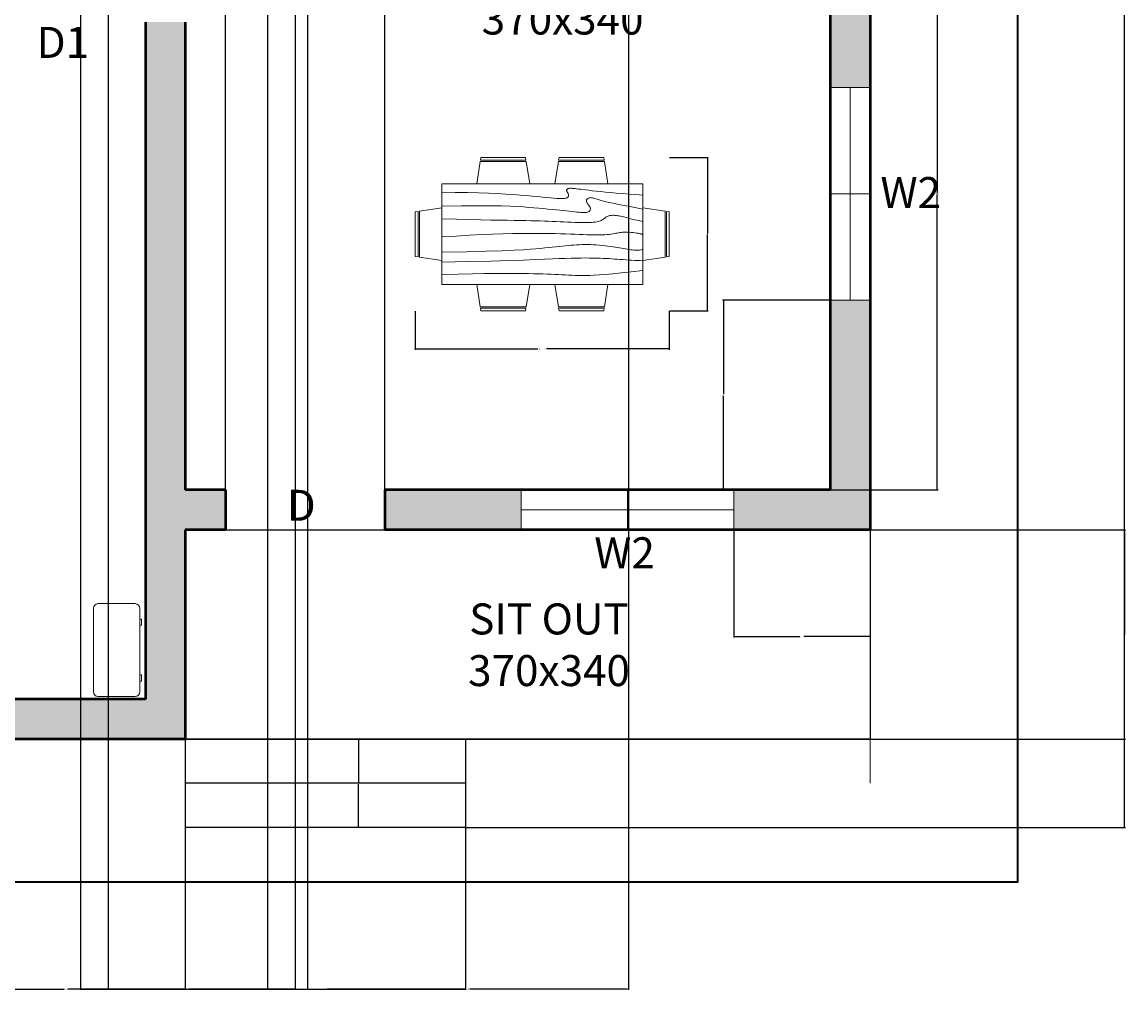
# Model space of a CAD drawing. Units: inches. Extents: x 5191 to 5616, y 7031 to 7539.
# Tile 2 of 4: x 5367 to 5616, y 7031 to 7250. Entities that reach past the tile are written whole.
import ezdxf

# ---------------------------------------------------------------- set-up
doc = ezdxf.new("R2010")
doc.units = ezdxf.units.IN
for name, color, linetype, lineweight in [('A-ANNO-DIMS', 2, 'Continuous', 13), ('A-ANNO-TEXT', 7, 'Continuous', 18), ('A-ANNO-TTLB', 7, 'Continuous', 35), ('A-AREA-IDEN', 7, 'Continuous', 25), ('A-FLOR-OTLN', 7, 'Continuous', 25), ('A-FLOR-STRS', 7, 'Continuous', 25), ('A-FURN', 8, 'Continuous', 18), ('A-GLAZ', 4, 'Continuous', 18), ('A-WALL', 7, 'Continuous', 50)]:
    doc.layers.add(name, color=color, linetype=linetype, lineweight=lineweight)
doc.layers.add('A-WALL-PATT', color=177, linetype='Continuous', lineweight=13, true_color=0x293189)
doc.styles.get("Standard").update_dxf_attribs({"font": 'arial.ttf'})
doc.dimstyles.get("Standard").update_dxf_attribs({"dimtxt": 0.18, "dimasz": 0.18, "dimexe": 0.18, "dimexo": 0.0625, "dimgap": 0.09, "dimtad": 0, "dimtih": 1, "dimtoh": 1, "dimdec": 4, "dimzin": 0, "dimdsep": 46, "dimtxsty": 'Standard', "dimcen": 0.09, "dimadec": 0, "dimazin": 0, "dimtfac": 1, "dimtdec": 4, "dimtofl": 0, "dimtmove": 0, "dimatfit": 3, "dimfxl": 1, "dimtolj": 1, "dimtzin": 0, "dimarcsym": 0})

# ---------------------------------------------------------------- blocks, each defined once
blk = doc.blocks.new('Dining Set - 36 x 72 in.')
for p, q in [((-22.2343, 26.00059), (-23.4847, 17.99762)), ((-22.2304, 26), (-5.7608, 26)), ((-22, 27.5), (-22.1562, 26.50042)), ((-5.8416, 26.5), (-22.1534, 26.5)), ((-22, 27.5), (-6, 27.5)), ((-5.8437, 26.49966), (-6, 27.5)), ((-4.5152, 17.99762), (-5.7655, 25.99926)), ((5.7657, 26.00059), (4.5153, 17.99762)), ((5.7696, 26), (22.2392, 26)), ((6, 27.5), (5.8438, 26.50042)), ((22.1584, 26.5), (5.8466, 26.5)), ((6, 27.5), (22, 27.5)), ((22.1563, 26.49966), (22, 27.5)), ((23.4848, 17.99762), (22.2345, 25.99926)), ((36, 18), (-36, 18)), ((-36, 18), (-36, -18)), ((36, -18), (36, 18)), ((-45.5, 8), (-44.5004, 8.15617)), ((-45.5, 8), (-45.5, -8)), ((-44.5, -8.15843), (-44.5, 8.15338)), ((-44.0006, 8.23428), (-35.9976, 9.48474)), ((-44, 8.23041), (-44, -8.23915)), ((44.0006, 8.23428), (35.9976, 9.48474)), ((44, 8.23041), (44, -8.23915)), ((44.5, -8.15843), (44.5, 8.15338)), ((45.5, 8), (44.5005, 8.15617)), ((45.5, 8), (45.5, -8)), ((-44.4997, -8.15631), (-45.5, -8)), ((-35.9976, -9.48476), (-43.9993, -8.2345)), ((35.9976, -9.48476), (43.9993, -8.2345)), ((44.4997, -8.15631), (45.5, -8)), ((-36, -18), (36, -18)), ((-22.2343, -26.0006), (-23.4847, -17.99762)), ((-4.5152, -17.99762), (-5.7655, -25.99928)), ((5.7657, -26.0006), (4.5153, -17.99762)), ((23.4848, -17.99762), (22.2345, -25.99928)), ((-22.2304, -26), (-5.7608, -26)), ((-22, -27.5), (-22.1562, -26.50044)), ((-5.8416, -26.5), (-22.1534, -26.5)), ((-22, -27.5), (-6, -27.5)), ((-5.8437, -26.49967), (-6, -27.5)), ((5.7696, -26), (22.2392, -26)), ((6, -27.5), (5.8438, -26.50044)), ((22.1584, -26.5), (5.8466, -26.5)), ((6, -27.5), (22, -27.5)), ((22.1563, -26.49967), (22, -27.5))]:
    blk.add_line(p, q)
for points in [[(-36, 15), (-31.1772, 14.97754), (-26.8079, 14.91406), (-22.8538, 14.81543), (-19.276, 14.6875), (-16.0362, 14.53613), (-13.0957, 14.36718), (-10.4159, 14.18652), (-7.9583, 14), (-5.6904, 13.81315), (-3.6035, 13.63021), (-1.6954, 13.45508), (0.0365, 13.29166), (1.5945, 13.14388), (2.9811, 13.01562), (4.1988, 12.9108), (5.25, 12.83333), (6.1393, 12.78613), (6.8802, 12.76823), (7.4883, 12.77767), (7.9792, 12.8125), (8.3685, 12.87077), (8.6719, 12.95052), (8.9049, 13.0498), (9.0833, 13.16666), (9.2205, 13.29899), (9.3216, 13.44401), (9.3895, 13.59879), (9.4271, 13.76041), (9.4373, 13.92594), (9.4232, 14.09245), (9.3875, 14.257), (9.3333, 14.41666), (9.2638, 14.56917), (9.1836, 14.71484), (9.0975, 14.85465), (9.0104, 14.98958), (8.9272, 15.1206), (8.8529, 15.2487), (8.7922, 15.37483), (8.75, 15.5), (8.7305, 15.62467), (8.7344, 15.74739), (8.7617, 15.86621), (8.8125, 15.97916), (8.8867, 16.08431), (8.9844, 16.17968), (9.1055, 16.26334), (9.25, 16.33333), (9.4189, 16.38802), (9.6172, 16.42708), (9.8506, 16.45052), (10.125, 16.45833), (10.4463, 16.45052), (10.8203, 16.42708), (11.2529, 16.38802), (11.75, 16.33333), (12.3184, 16.26318), (12.9694, 16.17838), (13.7151, 16.07991), (14.5677, 15.96875), (15.5395, 15.84586), (16.6426, 15.71224), (17.8893, 15.56884), (19.2917, 15.41666), (20.859, 15.25667), (22.5879, 15.08984), (24.4721, 14.91715), (26.5052, 14.73958), (28.6809, 14.5581), (30.9929, 14.3737), (33.4347, 14.18733), (36, 14)], [(-36, 10), (-28.9766, 10.14274), (-23.1725, 10.20442), (-18.4241, 10.19775), (-14.5677, 10.13541), (-11.4399, 10.03011), (-8.877, 9.89453), (-6.7154, 9.74137), (-4.7917, 9.58333), (-2.9698, 9.43082), (-1.2246, 9.28515), (0.4415, 9.14534), (2.026, 9.01041), (3.5266, 8.87939), (4.9408, 8.7513), (6.266, 8.62516), (7.5, 8.5), (8.6411, 8.37549), (9.6914, 8.2539), (10.6538, 8.13818), (11.5312, 8.03125), (12.3267, 7.93603), (13.043, 7.85547), (13.6831, 7.79248), (14.25, 7.75), (14.7471, 7.7303), (15.1797, 7.73307), (15.5537, 7.75732), (15.875, 7.80208), (16.1494, 7.86637), (16.3828, 7.94922), (16.5811, 8.04964), (16.75, 8.16666), (16.8944, 8.29915), (17.0143, 8.44531), (17.1089, 8.60319), (17.1771, 8.77083), (17.218, 8.94629), (17.2305, 9.1276), (17.2137, 9.31282), (17.1667, 9.5), (17.0895, 9.6875), (16.987, 9.875), (16.8649, 10.0625), (16.7292, 10.25), (16.5856, 10.4375), (16.4401, 10.625), (16.2985, 10.8125), (16.1667, 11), (16.05, 11.18733), (15.9518, 11.3737), (15.8752, 11.5581), (15.8229, 11.73958), (15.798, 11.91715), (15.8034, 12.08984), (15.842, 12.25667), (15.9167, 12.41666), (16.0295, 12.56836), (16.1784, 12.70833), (16.3605, 12.83268), (16.5729, 12.9375), (16.8127, 13.01888), (17.0768, 13.07291), (17.3625, 13.0957), (17.6667, 13.08333), (17.9894, 13.03312), (18.3418, 12.94726), (18.7382, 12.82918), (19.1927, 12.68229), (19.7195, 12.51001), (20.3327, 12.31575), (21.0465, 12.10294), (21.875, 11.875), (22.8357, 11.63354), (23.959, 11.37304), (25.2786, 11.08618), (26.8282, 10.76562), (28.6414, 10.40405), (30.752, 9.99414), (33.1936, 9.52856), (36, 9)], [(-36, 5.5), (-30.7157, 5.3348), (-26.069, 5.20963), (-21.9946, 5.11767), (-18.4271, 5.05208), (-15.3009, 5.00602), (-12.5508, 4.97265), (-10.1112, 4.94515), (-7.9167, 4.91666), (-5.909, 4.88167), (-4.0586, 4.83984), (-2.3429, 4.79215), (-0.7396, 4.73958), (0.7739, 4.6831), (2.22, 4.6237), (3.6213, 4.56233), (5, 4.5), (6.373, 4.43782), (7.7344, 4.3776), (9.0723, 4.32129), (10.375, 4.27083), (11.6309, 4.22819), (12.8281, 4.19531), (13.9551, 4.17415), (15, 4.16666), (15.954, 4.17448), (16.819, 4.19791), (17.6001, 4.23698), (18.3021, 4.29166), (18.9299, 4.36198), (19.4883, 4.44791), (19.9823, 4.54948), (20.4167, 4.66666), (20.7969, 4.79899), (21.1302, 4.94401), (21.4245, 5.09879), (21.6875, 5.26041), (21.9271, 5.42594), (22.1511, 5.59245), (22.3672, 5.757), (22.5834, 5.91666), (22.8065, 6.06868), (23.0404, 6.21093), (23.2879, 6.34147), (23.5521, 6.45833), (23.8358, 6.55957), (24.142, 6.64323), (24.4735, 6.70735), (24.8334, 6.75), (25.2235, 6.76969), (25.642, 6.76692), (26.0858, 6.74267), (26.5521, 6.69791), (27.0379, 6.63362), (27.5404, 6.55078), (28.0565, 6.45036), (28.5834, 6.33333), (29.1242, 6.19987), (29.7071, 6.04687), (30.3661, 5.87044), (31.1354, 5.66666), (32.0493, 5.43164), (33.142, 5.16146), (34.4475, 4.85221), (36, 4.5)], [(-36, -1), (-30.7915, -0.6591), (-26.0195, -0.38216), (-21.6519, -0.16284), (-17.6563, 0.00521), (-14.0005, 0.12833), (-10.6523, 0.21289), (-7.5796, 0.26522), (-4.75, 0.29166), (-2.134, 0.29793), (0.2878, 0.28711), (2.5317, 0.26163), (4.6146, 0.22396), (6.5529, 0.17651), (8.3633, 0.12174), (10.0623, 0.06209), (11.6667, 0), (13.1899, -0.06201), (14.6341, -0.1211), (15.9982, -0.17432), (17.2813, -0.21875), (18.4823, -0.25147), (19.6003, -0.26953), (20.6343, -0.27002), (21.5834, -0.25), (22.4481, -0.20768), (23.2357, -0.14584), (23.9549, -0.06836), (24.6146, 0.02083), (25.2235, 0.11784), (25.7904, 0.21875), (26.3241, 0.31966), (26.8334, 0.41666), (27.3265, 0.50618), (27.8099, 0.58593), (28.2894, 0.65397), (28.7709, 0.70833), (29.2601, 0.74707), (29.763, 0.76823), (30.2855, 0.76985), (30.8334, 0.75), (31.4088, 0.70784), (31.9994, 0.64713), (32.589, 0.57275), (33.1615, 0.48958), (33.7008, 0.4025), (34.1908, 0.3164), (34.6153, 0.23616), (34.9584, 0.16666), (35.2099, 0.11165), (35.3848, 0.07031), (35.504, 0.04069), (35.5886, 0.02083), (35.6594, 0.00879), (35.7377, 0.0026), (35.8442, 0.00032), (36, 0)], [(-36, -6.5), (-27.1843, -6.31267), (-20.084, -6.1263), (-14.469, -5.9419), (-10.1094, -5.76042), (-6.7752, -5.58285), (-4.2363, -5.41016), (-2.2629, -5.24333), (-0.625, -5.08334), (0.8708, -4.93099), (2.2715, -4.78646), (3.5872, -4.64974), (4.8281, -4.52084), (6.0046, -4.39974), (7.127, -4.28646), (8.2053, -4.18099), (9.25, -4.08334), (10.2705, -3.99382), (11.2734, -3.91407), (12.2647, -3.84603), (13.25, -3.79167), (14.2354, -3.75293), (15.2266, -3.73177), (16.2295, -3.73015), (17.25, -3.75), (18.2912, -3.79248), (19.3451, -3.85547), (20.4009, -3.93604), (21.4479, -4.03125), (22.4754, -4.13819), (23.4727, -4.25391), (24.4289, -4.37549), (25.3334, -4.5), (26.1785, -4.62492), (26.9694, -4.74935), (27.7145, -4.87281), (28.4219, -4.99479), (29.1, -5.11483), (29.7572, -5.23242), (30.4016, -5.34709), (31.0417, -5.45834), (31.6837, -5.56437), (32.3262, -5.65821), (32.9658, -5.73153), (33.599, -5.77604), (34.2224, -5.78345), (34.8327, -5.74545), (35.4264, -5.65373), (36, -5.5)], [(-36, -10), (-26.4022, -9.81299), (-18.4675, -9.62891), (-11.9839, -9.45069), (-6.7396, -9.28125), (-2.5226, -9.12354), (0.8789, -8.98047), (3.6769, -8.85498), (6.0833, -8.75), (8.2767, -8.66765), (10.3021, -8.60677), (12.1712, -8.56543), (13.8958, -8.54167), (15.4876, -8.53353), (16.9583, -8.53907), (18.3197, -8.55632), (19.5834, -8.58334), (20.7616, -8.61841), (21.8685, -8.66081), (22.9188, -8.71004), (23.9271, -8.76563), (24.9081, -8.82707), (25.8763, -8.89388), (26.8465, -8.96558), (27.8334, -9.04167), (28.8474, -9.12118), (29.8828, -9.20117), (30.93, -9.27824), (31.9792, -9.34896), (33.0205, -9.40991), (34.0443, -9.45768), (35.0407, -9.48885), (36, -9.5)], [(-36, -14.5), (-30.0881, -14.33513), (-25.0332, -14.21224), (-20.7312, -14.12647), (-17.0781, -14.07292), (-13.97, -14.04671), (-11.3027, -14.04297), (-8.9724, -14.05681), (-6.875, -14.08334), (-4.9224, -14.11833), (-3.0905, -14.16016), (-1.3709, -14.20785), (0.2448, -14.26042), (1.7647, -14.3169), (3.1973, -14.3763), (4.5507, -14.43767), (5.8333, -14.5), (7.0554, -14.5621), (8.235, -14.62175), (9.3922, -14.67652), (10.5469, -14.72396), (11.7192, -14.76164), (12.929, -14.78711), (14.1965, -14.79794), (15.5417, -14.79167), (16.9933, -14.76424), (18.6152, -14.70508), (20.4804, -14.60197), (22.6615, -14.44271), (25.2312, -14.21509), (28.2624, -13.9069), (31.8277, -13.50594), (36, -13)]]:
    blk.add_lwpolyline(points)
blk = doc.blocks.new('Desk - 30 x 60 in.')
for p, q in [((-26.999995, 0), (26.999995, 0)), ((-29.999995, -27), (-29.999995, -3)), ((29.999995, -3), (29.999995, -27)), ((26.999995, -30), (-26.999995, -30)), ((-20.000005, -30), (-20.000005, -31)), ((-20.000005, -31), (-16.000005, -31)), ((-16.000005, -31), (-16.000005, -30)), ((15.999995, -31), (15.999995, -30)), ((19.999995, -31), (15.999995, -31)), ((19.999995, -30), (19.999995, -31))]:
    blk.add_line(p, q)
for centre, start, end in [((-26.499995, -3.5), 98.1301, 171.8699), ((26.499995, -3.5), 8.130102, 81.8699), ((-26.499995, -26.5), 188.1301, 261.8699), ((26.499995, -26.5), 278.1301, 351.8699)]:
    blk.add_arc(centre, 3.535534, start, end)
blk = doc.blocks.new('WIN-W2-48IN')
for p, q in [((0, 0), (0, 9)), ((24, 0), (24, 9)), ((48, 0), (48, 9)), ((0, 4.5), (48, 4.5))]:
    blk.add_line(p, q)
blk = doc.blocks.new('*D23')
at = {"layer": 'A-ANNO-DIMS', "color": 0, "lineweight": -2, "transparency": 16777216}
for p, q in [((5455.33, 7184.28), (5455.33, 7175.56)), ((5512.71, 7184.28), (5512.71, 7175.56)), ((5455.51, 7175.74), (5483.05, 7175.74)), ((5512.53, 7175.74), (5484.99, 7175.74))]:
    blk.add_line(p, q, dxfattribs=at)
at = {"layer": 'A-ANNO-DIMS', "color": 0, "transparency": 16777216}
for points in [[(5455.51, 7175.77), (5455.51, 7175.71), (5455.33, 7175.74)], [(5512.53, 7175.77), (5512.53, 7175.71), (5512.71, 7175.74)]]:
    blk.add_solid(points, dxfattribs=at)
at = {"layer": 'Defpoints', "color": 0, "transparency": 16777216}
for p in [(5455.33, 7184.34), (5512.71, 7184.34), (5512.71, 7175.74)]:
    blk.add_point(p, dxfattribs=at)
at = {"layer": 'A-ANNO-DIMS', "color": 0, "transparency": 16777216, "insert": (5484.02, 7175.74), "char_height": 0.18, "attachment_point": 5}
blk.add_mtext('\\A1;DINING SET 57', dxfattribs=at)
blk = doc.blocks.new('*D24')
at = {"layer": 'A-ANNO-DIMS', "color": 0, "lineweight": -2, "transparency": 16777216}
for p, q in [((5512.77, 7219.03), (5521.5, 7219.03)), ((5521.32, 7218.85), (5521.32, 7201.87)), ((5521.32, 7184.52), (5521.32, 7201.5)), ((5512.77, 7184.34), (5521.5, 7184.34))]:
    blk.add_line(p, q, dxfattribs=at)
at = {"layer": 'A-ANNO-DIMS', "color": 0, "transparency": 16777216}
for points in [[(5521.29, 7218.85), (5521.35, 7218.85), (5521.32, 7219.03)], [(5521.29, 7184.52), (5521.35, 7184.52), (5521.32, 7184.34)]]:
    blk.add_solid(points, dxfattribs=at)
at = {"layer": 'Defpoints', "color": 0, "transparency": 16777216}
for p in [(5512.71, 7219.03), (5521.32, 7219.03), (5512.71, 7184.34)]:
    blk.add_point(p, dxfattribs=at)
at = {"layer": 'A-ANNO-DIMS', "color": 0, "transparency": 16777216, "insert": (5521.32, 7201.68), "char_height": 0.18, "attachment_point": 5}
blk.add_mtext('\\A1;35', dxfattribs=at)
blk = doc.blocks.new('*D32')
at = {"layer": 'A-ANNO-DIMS', "color": 0, "lineweight": -2, "transparency": 16777216}
for p, q in [((5428.24, 7514.77), (5615.71, 7514.77)), ((5615.53, 7514.59), (5615.53, 7291.37)), ((5615.53, 7067.79), (5615.53, 7291.01)), ((5466.73, 7067.61), (5615.71, 7067.61))]:
    blk.add_line(p, q, dxfattribs=at)
at = {"layer": 'A-ANNO-DIMS', "color": 0, "transparency": 16777216}
for points in [[(5615.5, 7514.59), (5615.56, 7514.59), (5615.53, 7514.77)], [(5615.5, 7067.79), (5615.56, 7067.79), (5615.53, 7067.61)]]:
    blk.add_solid(points, dxfattribs=at)
at = {"layer": 'Defpoints', "color": 0, "transparency": 16777216}
for p in [(5428.18, 7514.77), (5615.53, 7514.77), (5466.67, 7067.61)]:
    blk.add_point(p, dxfattribs=at)
at = {"layer": 'A-ANNO-DIMS', "color": 0, "transparency": 16777216, "insert": (5615.53, 7291.19), "char_height": 0.18, "attachment_point": 5}
blk.add_mtext('\\A1;447.2', dxfattribs=at)
blk = doc.blocks.new('*D34')
at = {"layer": 'A-ANNO-DIMS', "color": 0, "lineweight": -2, "transparency": 16777216}
for p, q in [((5349.51, 7087.55), (5349.51, 7030.92)), ((5403.39, 7087.55), (5403.39, 7030.92)), ((5349.69, 7031.1), (5376.06, 7031.1)), ((5403.21, 7031.1), (5376.84, 7031.1))]:
    blk.add_line(p, q, dxfattribs=at)
at = {"layer": 'A-ANNO-DIMS', "color": 0, "transparency": 16777216}
for points in [[(5349.69, 7031.13), (5349.69, 7031.07), (5349.51, 7031.1)], [(5403.21, 7031.13), (5403.21, 7031.07), (5403.39, 7031.1)]]:
    blk.add_solid(points, dxfattribs=at)
at = {"layer": 'Defpoints', "color": 0, "transparency": 16777216}
for p in [(5349.51, 7087.61), (5403.39, 7087.61), (5403.39, 7031.1)]:
    blk.add_point(p, dxfattribs=at)
at = {"layer": 'A-ANNO-DIMS', "color": 0, "transparency": 16777216, "insert": (5376.45, 7031.1), "char_height": 0.18, "attachment_point": 5}
blk.add_mtext('\\A1;53.88', dxfattribs=at)
blk = doc.blocks.new('*D35')
at = {"layer": 'A-ANNO-DIMS', "color": 0, "lineweight": -2, "transparency": 16777216}
for p, q in [((5403.39, 7067.55), (5403.39, 7030.92)), ((5466.67, 7067.55), (5466.67, 7030.92)), ((5403.57, 7031.1), (5434.63, 7031.1)), ((5466.49, 7031.1), (5435.42, 7031.1))]:
    blk.add_line(p, q, dxfattribs=at)
at = {"layer": 'A-ANNO-DIMS', "color": 0, "transparency": 16777216}
for points in [[(5403.57, 7031.13), (5403.57, 7031.07), (5403.39, 7031.1)], [(5466.49, 7031.13), (5466.49, 7031.07), (5466.67, 7031.1)]]:
    blk.add_solid(points, dxfattribs=at)
at = {"layer": 'Defpoints', "color": 0, "transparency": 16777216}
for p in [(5403.39, 7067.61), (5466.67, 7067.61), (5466.67, 7031.1)]:
    blk.add_point(p, dxfattribs=at)
at = {"layer": 'A-ANNO-DIMS', "color": 0, "transparency": 16777216, "insert": (5435.03, 7031.1), "char_height": 0.18, "attachment_point": 5}
blk.add_mtext('\\A1;63.28', dxfattribs=at)
blk = doc.blocks.new('*D36')
at = {"layer": 'A-ANNO-DIMS', "color": 0, "lineweight": -2, "transparency": 16777216}
for p, q in [((5466.6, 7087.61), (5442.34, 7087.61)), ((5442.52, 7087.43), (5442.52, 7077.8)), ((5442.52, 7067.79), (5442.52, 7077.43)), ((5466.6, 7067.61), (5442.34, 7067.61))]:
    blk.add_line(p, q, dxfattribs=at)
at = {"layer": 'A-ANNO-DIMS', "color": 0, "transparency": 16777216}
for points in [[(5442.49, 7087.43), (5442.55, 7087.43), (5442.52, 7087.61)], [(5442.49, 7067.79), (5442.55, 7067.79), (5442.52, 7067.61)]]:
    blk.add_solid(points, dxfattribs=at)
at = {"layer": 'Defpoints', "color": 0, "transparency": 16777216}
for p in [(5442.52, 7087.61), (5466.67, 7087.61), (5466.67, 7067.61)]:
    blk.add_point(p, dxfattribs=at)
at = {"layer": 'A-ANNO-DIMS', "color": 0, "transparency": 16777216, "insert": (5442.52, 7077.61), "char_height": 0.18, "attachment_point": 5}
blk.add_mtext('\\A1;20', dxfattribs=at)
blk = doc.blocks.new('*D38')
at = {"layer": 'A-ANNO-DIMS', "color": 0, "lineweight": -2, "transparency": 16777216}
for p, q in [((5379.71, 7504.71), (5379.71, 7030.92)), ((5428.18, 7504.71), (5428.18, 7030.92)), ((5379.89, 7031.1), (5403.55, 7031.1)), ((5428, 7031.1), (5404.34, 7031.1))]:
    blk.add_line(p, q, dxfattribs=at)
at = {"layer": 'A-ANNO-DIMS', "color": 0, "transparency": 16777216}
for points in [[(5379.89, 7031.13), (5379.89, 7031.07), (5379.71, 7031.1)], [(5428, 7031.13), (5428, 7031.07), (5428.18, 7031.1)]]:
    blk.add_solid(points, dxfattribs=at)
at = {"layer": 'Defpoints', "color": 0, "transparency": 16777216}
for p in [(5379.71, 7504.77), (5428.18, 7504.77), (5428.18, 7031.1)]:
    blk.add_point(p, dxfattribs=at)
at = {"layer": 'A-ANNO-DIMS', "color": 0, "transparency": 16777216, "insert": (5403.95, 7031.1), "char_height": 0.18, "attachment_point": 5}
blk.add_mtext('\\A1;48.47', dxfattribs=at)
blk = doc.blocks.new('*D42')
at = {"layer": 'A-ANNO-DIMS', "color": 0, "lineweight": -2, "transparency": 16777216}
for p, q in [((5403.45, 7134.89), (5615.71, 7134.89)), ((5615.53, 7134.71), (5615.53, 7111.44)), ((5615.53, 7087.79), (5615.53, 7111.07)), ((5403.45, 7087.61), (5615.71, 7087.61))]:
    blk.add_line(p, q, dxfattribs=at)
at = {"layer": 'A-ANNO-DIMS', "color": 0, "transparency": 16777216}
for points in [[(5615.5, 7134.71), (5615.56, 7134.71), (5615.53, 7134.89)], [(5615.5, 7087.79), (5615.56, 7087.79), (5615.53, 7087.61)]]:
    blk.add_solid(points, dxfattribs=at)
at = {"layer": 'Defpoints', "color": 0, "transparency": 16777216}
for p in [(5403.39, 7134.89), (5615.53, 7134.89), (5403.39, 7087.61)]:
    blk.add_point(p, dxfattribs=at)
at = {"layer": 'A-ANNO-DIMS', "color": 0, "transparency": 16777216, "insert": (5615.53, 7111.25), "char_height": 0.18, "attachment_point": 5}
blk.add_mtext('\\A1;47.28', dxfattribs=at)
blk = doc.blocks.new('*D43')
at = {"layer": 'A-ANNO-DIMS', "color": 0, "lineweight": -2, "transparency": 16777216}
for p, q in [((5549.01, 7186.79), (5524.74, 7186.79)), ((5524.92, 7186.61), (5524.92, 7165.53)), ((5524.92, 7144.07), (5524.92, 7165.16)), ((5549.01, 7143.89), (5524.74, 7143.89))]:
    blk.add_line(p, q, dxfattribs=at)
at = {"layer": 'A-ANNO-DIMS', "color": 0, "transparency": 16777216}
for points in [[(5524.89, 7186.61), (5524.95, 7186.61), (5524.92, 7186.79)], [(5524.89, 7144.07), (5524.95, 7144.07), (5524.92, 7143.89)]]:
    blk.add_solid(points, dxfattribs=at)
at = {"layer": 'Defpoints', "color": 0, "transparency": 16777216}
for p in [(5524.92, 7186.79), (5549.07, 7186.79), (5549.07, 7143.89)]:
    blk.add_point(p, dxfattribs=at)
at = {"layer": 'A-ANNO-DIMS', "color": 0, "transparency": 16777216, "insert": (5524.92, 7165.34), "char_height": 0.18, "attachment_point": 5}
blk.add_mtext('\\A1;42.9', dxfattribs=at)
blk = doc.blocks.new('*D44')
at = {"layer": 'A-ANNO-DIMS', "color": 0, "lineweight": -2, "transparency": 16777216}
for p, q in [((5549.13, 7277.69), (5573.4, 7277.69)), ((5573.22, 7277.51), (5573.22, 7210.98)), ((5573.22, 7144.07), (5573.22, 7210.61)), ((5549.13, 7143.89), (5573.4, 7143.89))]:
    blk.add_line(p, q, dxfattribs=at)
at = {"layer": 'A-ANNO-DIMS', "color": 0, "transparency": 16777216}
for points in [[(5573.19, 7277.51), (5573.25, 7277.51), (5573.22, 7277.69)], [(5573.19, 7144.07), (5573.25, 7144.07), (5573.22, 7143.89)]]:
    blk.add_solid(points, dxfattribs=at)
at = {"layer": 'Defpoints', "color": 0, "transparency": 16777216}
for p in [(5549.07, 7277.69), (5549.07, 7143.89), (5573.22, 7143.89)]:
    blk.add_point(p, dxfattribs=at)
at = {"layer": 'A-ANNO-DIMS', "color": 0, "transparency": 16777216, "insert": (5573.22, 7210.79), "char_height": 0.18, "attachment_point": 5}
blk.add_mtext('\\A1;133.8', dxfattribs=at)
blk = doc.blocks.new('*D49')
at = {"layer": 'A-ANNO-DIMS', "color": 0, "lineweight": -2, "transparency": 16777216}
for p, q in [((5385.99, 7494.71), (5385.99, 7030.92)), ((5421.99, 7494.71), (5421.99, 7030.92)), ((5386.17, 7031.1), (5403.77, 7031.1)), ((5421.81, 7031.1), (5404.21, 7031.1))]:
    blk.add_line(p, q, dxfattribs=at)
at = {"layer": 'A-ANNO-DIMS', "color": 0, "transparency": 16777216}
for points in [[(5386.17, 7031.13), (5386.17, 7031.07), (5385.99, 7031.1)], [(5421.81, 7031.13), (5421.81, 7031.07), (5421.99, 7031.1)]]:
    blk.add_solid(points, dxfattribs=at)
at = {"layer": 'Defpoints', "color": 0, "transparency": 16777216}
for p in [(5385.99, 7494.77), (5421.99, 7494.77), (5421.99, 7031.1)]:
    blk.add_point(p, dxfattribs=at)
at = {"layer": 'A-ANNO-DIMS', "color": 0, "transparency": 16777216, "insert": (5403.99, 7031.1), "char_height": 0.18, "attachment_point": 5}
blk.add_mtext('\\A1;36', dxfattribs=at)
blk = doc.blocks.new('*D51')
at = {"layer": 'A-ANNO-DIMS', "color": 0, "lineweight": -2, "transparency": 16777216}
for p, q in [((5412.46, 7143.96), (5412.46, 7539.1)), ((5448.46, 7143.96), (5448.46, 7539.1)), ((5412.64, 7538.92), (5430.24, 7538.92)), ((5448.28, 7538.92), (5430.68, 7538.92))]:
    blk.add_line(p, q, dxfattribs=at)
at = {"layer": 'A-ANNO-DIMS', "color": 0, "transparency": 16777216}
for points in [[(5412.64, 7538.95), (5412.64, 7538.89), (5412.46, 7538.92)], [(5448.28, 7538.95), (5448.28, 7538.89), (5448.46, 7538.92)]]:
    blk.add_solid(points, dxfattribs=at)
at = {"layer": 'Defpoints', "color": 0, "transparency": 16777216}
for p in [(5448.46, 7538.92), (5412.46, 7143.89), (5448.46, 7143.89)]:
    blk.add_point(p, dxfattribs=at)
at = {"layer": 'A-ANNO-DIMS', "color": 0, "transparency": 16777216, "insert": (5430.46, 7538.92), "char_height": 0.18, "attachment_point": 5}
blk.add_mtext('\\A1;36', dxfattribs=at)
blk = doc.blocks.new('*D52')
at = {"layer": 'A-ANNO-DIMS', "color": 0, "lineweight": -2, "transparency": 16777216}
for p, q in [((5527.27, 7134.83), (5527.27, 7110.56)), ((5558.07, 7134.83), (5558.07, 7110.56)), ((5527.45, 7110.74), (5542.2, 7110.74)), ((5557.89, 7110.74), (5543.13, 7110.74))]:
    blk.add_line(p, q, dxfattribs=at)
at = {"layer": 'A-ANNO-DIMS', "color": 0, "transparency": 16777216}
for points in [[(5527.45, 7110.77), (5527.45, 7110.71), (5527.27, 7110.74)], [(5557.89, 7110.77), (5557.89, 7110.71), (5558.07, 7110.74)]]:
    blk.add_solid(points, dxfattribs=at)
at = {"layer": 'Defpoints', "color": 0, "transparency": 16777216}
for p in [(5527.27, 7134.89), (5558.07, 7134.89), (5527.27, 7110.74)]:
    blk.add_point(p, dxfattribs=at)
at = {"layer": 'A-ANNO-DIMS', "color": 0, "transparency": 16777216, "insert": (5542.67, 7110.74), "char_height": 0.18, "attachment_point": 5}
blk.add_mtext('\\A1;30.806', dxfattribs=at)
blk = doc.blocks.new('*D54')
at = {"layer": 'A-ANNO-DIMS', "color": 0, "lineweight": -2, "transparency": 16777216}
for p, q in [((5430.99, 7421.63), (5430.99, 7030.92)), ((5503.47, 7421.63), (5503.47, 7030.92)), ((5431.17, 7031.1), (5466.84, 7031.1)), ((5503.29, 7031.1), (5467.62, 7031.1))]:
    blk.add_line(p, q, dxfattribs=at)
at = {"layer": 'A-ANNO-DIMS', "color": 0, "transparency": 16777216}
for points in [[(5431.17, 7031.13), (5431.17, 7031.07), (5430.99, 7031.1)], [(5503.29, 7031.13), (5503.29, 7031.07), (5503.47, 7031.1)]]:
    blk.add_solid(points, dxfattribs=at)
at = {"layer": 'Defpoints', "color": 0, "transparency": 16777216}
for p in [(5430.99, 7421.69), (5503.47, 7421.69), (5503.47, 7031.1)]:
    blk.add_point(p, dxfattribs=at)
at = {"layer": 'A-ANNO-DIMS', "color": 0, "transparency": 16777216, "insert": (5467.23, 7031.1), "char_height": 0.18, "attachment_point": 5}
blk.add_mtext('\\A1;72.48', dxfattribs=at)

msp = doc.modelspace()

# ---------------------------------------------------------------- hatches: boundary and pattern name
at = {"layer": 'A-WALL-PATT'}
h = msp.add_hatch(color=256, dxfattribs=at)
h.dxf.hatch_style = 1
h.paths.add_polyline_path([(5297.311, 7494.7733), (5247.631, 7494.7733), (5247.631, 7441.5533), (5256.631, 7441.5533), (5256.631, 7485.7733), (5297.311, 7485.7733)])
h.paths.add_polyline_path([(5503.471, 7430.6933), (5503.471, 7461.7733), (5494.471, 7461.7733), (5494.471, 7430.6933), (5430.991, 7430.6933), (5430.991, 7485.7733), (5450.731, 7485.7733), (5450.731, 7494.7733), (5421.991, 7494.7733), (5421.991, 7485.7733), (5421.991, 7337.3333), (5421.991, 7328.3333), (5430.991, 7328.3333), (5430.991, 7337.3333), (5430.991, 7421.6933), (5503.471, 7421.6933)])
h.paths.add_polyline_path([(5385.991, 7494.7733), (5345.311, 7494.7733), (5345.311, 7485.7733), (5385.991, 7485.7733)])
h.paths.add_polyline_path([(5558.071, 7494.7733), (5474.731, 7494.7733), (5474.731, 7485.7733), (5494.471, 7485.7733), (5503.471, 7485.7733), (5549.071, 7485.7733), (5549.071, 7397.3333), (5558.071, 7397.3333)])
h.paths.add_polyline_path([(5385.991, 7337.3333), (5256.631, 7337.3333), (5256.631, 7381.5533), (5247.631, 7381.5533), (5247.631, 7337.3333), (5247.631, 7328.3333), (5247.631, 7300.9733), (5256.631, 7300.9733), (5256.631, 7328.3333), (5385.991, 7328.3333)])
h.paths.add_polyline_path([(5358.391, 7249.6133), (5303.911, 7249.6133), (5256.631, 7249.6133), (5256.631, 7276.9733), (5247.631, 7276.9733), (5247.631, 7249.6133), (5247.631, 7240.6133), (5247.631, 7207.6133), (5256.631, 7207.6133), (5256.631, 7240.6133), (5303.911, 7240.6133), (5358.391, 7240.6133)])
h.paths.add_polyline_path([(5256.631, 7114.6133), (5256.631, 7147.6133), (5247.631, 7147.6133), (5247.631, 7114.6133), (5247.631, 7105.6133), (5247.631, 7087.6133), (5301.511, 7087.6133), (5301.511, 7096.6133), (5256.631, 7096.6133)])
h.paths.add_polyline_path([(5403.391, 7105.6133), (5403.391, 7114.6133), (5403.391, 7134.8933), (5412.4598, 7134.8933), (5412.4598, 7143.8933), (5403.391, 7143.8933), (5403.391, 7249.6133), (5394.391, 7249.6133), (5394.391, 7143.8933), (5394.391, 7134.8933), (5394.391, 7114.6133), (5394.391, 7096.6133), (5349.511, 7096.6133), (5349.511, 7087.6133), (5403.391, 7087.6133)])
h.paths.add_polyline_path([(5558.071, 7143.8933), (5558.071, 7186.7933), (5549.071, 7186.7933), (5549.071, 7143.8933), (5527.2654, 7143.8933), (5527.2654, 7134.8933), (5558.071, 7134.8933)])
h.paths.add_polyline_path([(5479.2654, 7143.8933), (5448.4598, 7143.8933), (5448.4598, 7134.8933), (5479.2654, 7134.8933)])
h.paths.add_polyline_path([(5558.071, 7337.3333), (5549.071, 7337.3333), (5549.071, 7286.6933), (5421.991, 7286.6933), (5421.991, 7277.6933), (5430.991, 7277.6933), (5549.071, 7277.6933), (5549.071, 7234.7933), (5558.071, 7234.7933), (5558.071, 7277.6933)])

# ---------------------------------------------------------------- linework, layer by layer
at = {"layer": 'A-ANNO-DIMS'}
for p, q in [((5558.071, 7134.8933), (5568.071, 7134.8933)), ((5558.071, 7087.6133), (5558.071, 7077.6133))]:
    msp.add_line(p, q, dxfattribs=at)
at = {"layer": 'A-ANNO-TTLB'}
msp.add_lwpolyline([(5215.7388, 7536.9841), (5591.3795, 7536.9841), (5591.3795, 7055.2452), (5215.7388, 7055.2452)], close=True, dxfattribs=at)
at = {"layer": 'A-FLOR-OTLN'}
for p, q in [((5558.071, 7134.8933), (5558.071, 7087.6133)), ((5558.071, 7087.6133), (5403.391, 7087.6133))]:
    msp.add_line(p, q, dxfattribs=at)
at = {"layer": 'A-FLOR-STRS'}
for p, q in [((5403.391, 7087.6133), (5403.391, 7067.6133)), ((5466.6673, 7087.6133), (5466.6673, 7067.6133)), ((5466.6673, 7077.6133), (5403.391, 7077.6133)), ((5466.6673, 7067.6133), (5403.391, 7067.6133))]:
    msp.add_line(p, q, dxfattribs=at)
at = {"layer": 'A-WALL'}
for p, q in [((5549.071, 7277.6933), (5549.071, 7143.8933)), ((5558.071, 7277.6933), (5558.071, 7143.8933)), ((5394.391, 7249.6133), (5394.391, 7143.8933)), ((5403.391, 7249.6133), (5403.391, 7143.8933)), ((5394.391, 7143.8933), (5394.391, 7134.8933)), ((5412.4598, 7143.8933), (5403.391, 7143.8933)), ((5412.4598, 7143.8933), (5412.4598, 7134.8933)), ((5549.071, 7143.8933), (5448.4598, 7143.8933)), ((5448.4598, 7143.8933), (5448.4598, 7134.8933)), ((5558.071, 7143.8933), (5558.071, 7134.8933)), ((5394.391, 7134.8933), (5394.391, 7114.6133)), ((5403.391, 7134.8933), (5403.391, 7114.6133)), ((5412.4598, 7134.8933), (5403.391, 7134.8933)), ((5558.071, 7134.8933), (5448.4598, 7134.8933)), ((5394.391, 7114.6133), (5394.391, 7096.6133)), ((5403.391, 7114.6133), (5403.391, 7105.6133)), ((5403.391, 7105.6133), (5403.391, 7087.6133)), ((5394.391, 7096.6133), (5256.631, 7096.6133)), ((5403.391, 7087.6133), (5247.631, 7087.6133))]:
    msp.add_line(p, q, dxfattribs=at)

# ---------------------------------------------------------------- block references
at = {"layer": 'A-FURN', "xscale": 0.6305744962266285, "yscale": 0.6305744962266285, "zscale": 0.6305744962266285}
msp.add_blockref('Dining Set - 36 x 72 in.', (5484.0175, 7201.6843), dxfattribs=at)
at = {"layer": 'A-FURN', "xscale": 0.350301795417789, "yscale": 0.350301795417789, "zscale": 0.350301795417789, "rotation": 89.99999999999999}
msp.add_blockref('Desk - 30 x 60 in.', (5382.6324, 7107.7082), dxfattribs=at)
at = {"layer": 'A-GLAZ'}
for p, rotation in [((5558.0713, 7186.7933), 90.0000000000067), ((5527.2654, 7143.8936), 180)]:
    msp.add_blockref('WIN-W2-48IN', p, dxfattribs=dict(at, rotation=rotation))

# ---------------------------------------------------------------- texts
at = {"layer": 'A-ANNO-TEXT', "char_height": 7, "attachment_point": 1}
for s, width, insert in [('\\pxqc;D1', 18.543886, (5366.4732, 7248.5149)), ('\\pxqc;W2', 29.703042, (5552.388, 7214.5926)), ('\\pxqc;D', 19.531951, (5419.7934, 7143.9297)), ('\\pxqc;W2', 29.703042, (5487.7477, 7133.1955))]:
    msp.add_mtext_dynamic_manual_height_columns(s, width=width, gutter_width=12.5, heights=[0], dxfattribs=dict(at, insert=insert))
at = {"layer": 'A-AREA-IDEN', "char_height": 7, "attachment_point": 1}
for s, width, insert in [('\\pxqc;{\\fArial|b1|i0|c0|p34;LIVING & DINNING\\P370x340}', 103.767041, (5436.7343, 7265.4722)), ('\\pxqc;{\\fArial|b1|i0|c0|p34;SIT OUT\\P370x340}', 73.840463, (5448.6206, 7118.2435))]:
    msp.add_mtext_dynamic_manual_height_columns(s, width=width, gutter_width=12.5, heights=[0], dxfattribs=dict(at, insert=insert))

# ---------------------------------------------------------------- dimensions: what is measured, and where the dimension line sits
at = {"layer": 'A-ANNO-DIMS'}
for base, p1, p2, override, picture, middle in [((5448.4598, 7538.9233), (5412.4598, 7143.8933), (5448.4598, 7143.8933), {"dimdec": 0, "dimlfac": 1, "dimrnd": 0, "dimzin": 0, "dimdsep": 46, "dimlunit": 2}, '*D51', (5430.4598, 7538.9233)), ((5428.1805, 7031.0952), (5379.7136, 7504.7733), (5428.1805, 7504.7733), {"dimdec": 2, "dimlfac": 1, "dimrnd": 0, "dimzin": 0, "dimdsep": 46, "dimlunit": 2}, '*D38', (5403.947, 7031.0952)), ((5421.991, 7031.0952), (5385.991, 7494.7733), (5421.991, 7494.7733), {"dimdec": 0, "dimlfac": 1, "dimrnd": 0, "dimzin": 0, "dimdsep": 46, "dimlunit": 2}, '*D49', (5403.991, 7031.0952)), ((5503.471, 7031.0952), (5430.991, 7421.6933), (5503.471, 7421.6933), {"dimdec": 2, "dimlfac": 1, "dimrnd": 0, "dimzin": 0, "dimdsep": 46, "dimlunit": 2}, '*D54', (5467.231, 7031.0952)), ((5403.391, 7031.0952), (5349.511, 7087.6133), (5403.391, 7087.6133), {"dimdec": 2, "dimlfac": 1, "dimrnd": 0, "dimzin": 0, "dimdsep": 46, "dimlunit": 2}, '*D34', (5376.451, 7031.0952)), ((5466.6673, 7031.0952), (5403.391, 7067.6133), (5466.6673, 7067.6133), {"dimdec": 2, "dimlfac": 1, "dimrnd": 0, "dimzin": 0, "dimdsep": 46, "dimlunit": 2}, '*D35', (5435.0291, 7031.0952))]:
    dim = msp.add_linear_dim(base=base, p1=p1, p2=p2, dimstyle='Standard', override=override, dxfattribs=at)
    dim.commit()
    dim.dimension.update_dxf_attribs({"geometry": picture, "text_midpoint": middle})
for base, p1, p2, angle, override, picture, middle in [((5615.5295, 7514.7733), (5466.6673, 7067.6133), (5428.1805, 7514.7733), 90, {"dimdec": 1, "dimlfac": 1, "dimrnd": 0, "dimzin": 0, "dimdsep": 46, "dimlunit": 2}, '*D32', (5615.5295, 7291.1933)), ((5573.221, 7143.8933), (5549.071, 7277.6933), (5549.071, 7143.8933), 270, {"dimdec": 1, "dimlfac": 1, "dimrnd": 0, "dimzin": 0, "dimdsep": 46, "dimlunit": 2}, '*D44', (5573.221, 7210.7933)), ((5521.316, 7219.0251), (5512.7087, 7184.3435), (5512.7087, 7219.0251), 90, {"dimdec": 0, "dimlfac": 1, "dimrnd": 0, "dimzin": 0, "dimdsep": 46, "dimlunit": 2}, '*D24', (5521.316, 7201.6843)), ((5524.921, 7186.7933), (5549.071, 7143.8933), (5549.071, 7186.7933), 90, {"dimdec": 1, "dimlfac": 1, "dimrnd": 0, "dimzin": 0, "dimdsep": 46, "dimlunit": 2}, '*D43', (5524.921, 7165.3433)), ((5615.5295, 7134.8933), (5403.391, 7087.6133), (5403.391, 7134.8933), 90, {"dimdec": 2, "dimlfac": 1, "dimrnd": 0, "dimzin": 0, "dimdsep": 46, "dimlunit": 2}, '*D42', (5615.5295, 7111.2533)), ((5527.2654, 7110.7433), (5558.071, 7134.8933), (5527.2654, 7134.8933), 180, {"dimdec": 3, "dimlfac": 1, "dimrnd": 0, "dimzin": 0, "dimdsep": 46, "dimlunit": 2}, '*D52', (5542.6682, 7110.7433)), ((5442.5173, 7087.6133), (5466.6673, 7067.6133), (5466.6673, 7087.6133), 90, {"dimdec": 0, "dimlfac": 1, "dimrnd": 0, "dimzin": 0, "dimdsep": 46, "dimlunit": 2}, '*D36', (5442.5173, 7077.6133))]:
    dim = msp.add_linear_dim(base=base, p1=p1, p2=p2, angle=angle, dimstyle='Standard', override=override, dxfattribs=at)
    dim.commit()
    dim.dimension.update_dxf_attribs({"geometry": picture, "text_midpoint": middle})
dim = msp.add_linear_dim(base=(5512.7087, 7175.7362), p1=(5455.3264, 7184.3435), p2=(5512.7087, 7184.3435), text='DINING SET <>', dimstyle='Standard', override={"dimdec": 0, "dimlfac": 1, "dimrnd": 0, "dimzin": 0, "dimdsep": 46, "dimlunit": 2}, dxfattribs=at)
dim.commit()
dim.dimension.update_dxf_attribs({"geometry": '*D23', "text_midpoint": (5484.0175, 7175.7362)})

doc.saveas('drawing.dxf')
